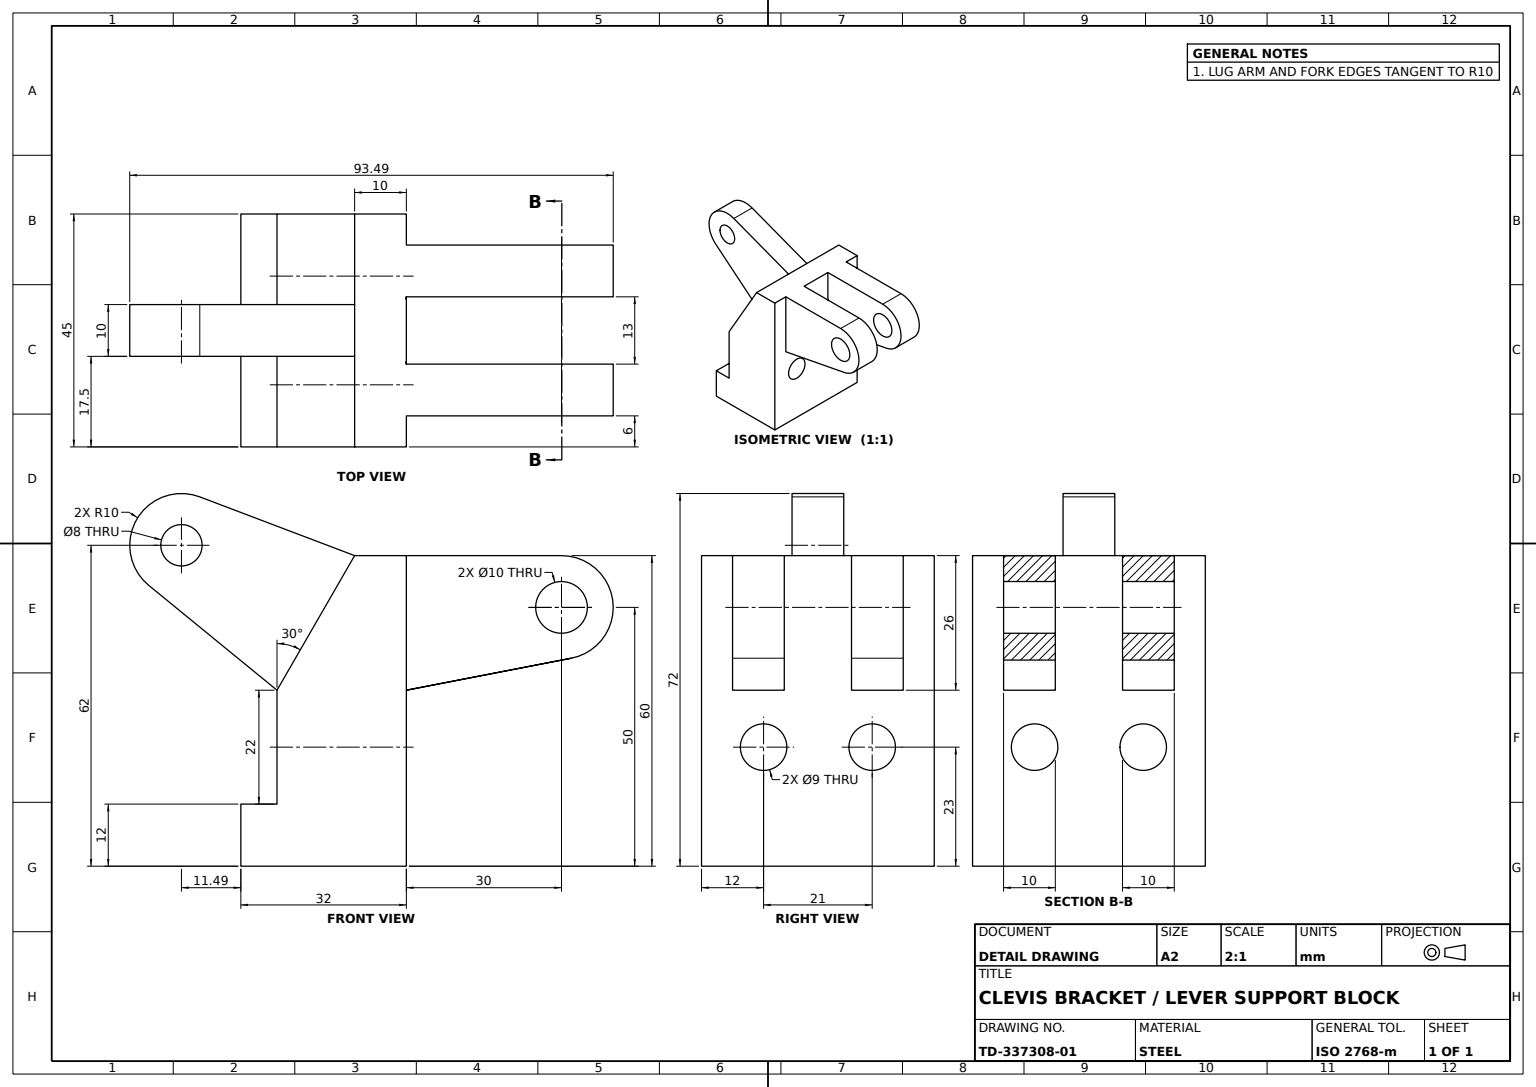
SolidWorks part; units mm, degrees
material "Plain Carbon Steel"
ref_plane "Front Plane" through (0, 0, 0) normal (0, 0, 1) x (1, 0, 0)
ref_plane "Top Plane" through (0, 0, 0) normal (0, 1, 0) x (1, 0, 0)
ref_plane "Right Plane" through (0, 0, 0) normal (1, 0, 0) x (0, 0, -1)
sketch "Base Block Profile Sketch" plane through (0, 0, 0) normal (0, 0, 1) x (1, 0, 0)
  line L0 (0, 0) -> (-32, 0)
  line L1 (-32, 0) -> (-32, 12)
  line L2 (-32, 12) -> (-25.0111, 12)
  line L3 (-25.0111, 12) -> (-25.0111, 34)
  line L4 (-25.0111, 34) -> (-10, 60)
  line L5 (-10, 60) -> (0, 60)
  line L6 (0, 60) -> (0, 0)
  dimension "D1" = 10
  dimension "D2" = 60
  dimension "D3" = 32
  dimension "D4" = 12
  dimension "D5" = 22
  dimension "D6" = 30
extrude "Base Block" add sketch "Base Block Profile Sketch" along normal mid plane 45
sketch "Lug Arm Sketch" plane through (0, 0, 0) normal (0, 0, 1) x (1, 0, 0)
  line L0 (-25.0111, 34) -> (-49.8118, 54.2548)
  line L1 (-43.4863, 62) -> (-17.5056, 47) construction
  line L2 (-10, 60) -> (-25.0111, 34) construction
  line L3 (-39.9415, 71.3506) -> (-10, 60)
  line L4 (-25.0111, 34) -> (-10, 60)
  arc A0 (-39.9415, 71.3506) -> (-49.8118, 54.2548) centre (-43.4863, 62) ccw
  circle A1 centre (-43.4863, 62) radius 4
  point P5 (-17.5056, 47)
  dimension "D2" = 8
  dimension "D3" = 10
  dimension "D1" = 30
extrude "Lug Arm" add sketch "Lug Arm Sketch" along normal mid plane 10
sketch "Side Hole Sketch" plane through (-25.0111, 0, 0) normal (-1, 0, 0) x (0, 0, 1)
  line L0 (22.5, 34) -> (22.5, 12) construction
  circle A0 centre (10.5, 23) radius 4.5
  circle A1 centre (-10.5, 23) radius 4.5
  point P8 (22.5, 23)
  dimension "D1" = 9
  dimension "D2" = 21
  dimension "D3" = 10.5
extrude "Side Hole Ø9" cut sketch "Side Hole Sketch" against normal up to next
sketch "Clevis Fork Sketch" plane through (0, 0, 22.5) normal (0, 0, 1) x (1, 0, 0)
  line L0 (0, 60) -> (30, 60)
  line L1 (0, 34) -> (31.9026, 40.1827)
  line L2 (0, 0) -> (0, 60) construction
  line L3 (0, 60) -> (0, 34)
  arc A0 (31.9026, 40.1827) -> (30, 60) centre (30, 50) ccw
  circle A1 centre (30, 50) radius 5
  dimension "D1" = 20
  dimension "D3" = 10
  dimension "D2" = 26
  dimension "D4" = 30
extrude "Clevis Fork" add sketch "Clevis Fork Sketch" against normal up to surface (45 mm away) up to face at (-17.7175, 25.4286, -22.5)
sketch "Clevis Pin Hole Sketch" plane through (0, 60, 0) normal (0, 1, 0) x (1, 0, 0)
  line L0 (0, 22.5) -> (0, -22.5) construction
  line L1 (0, -16.5) -> (40, -16.5)
  line L2 (0, -16.5) -> (0, -22.5)
  line L3 (0, -22.5) -> (40, -22.5)
  line L4 (40, -16.5) -> (40, -22.5)
  line L5 (40, -22.5) -> (40, 22.5) construction
  line L6 (30, -22.5) -> (-10, -22.5) construction
  line L7 (0, -6.5) -> (40, -6.5)
  line L8 (0, -6.5) -> (0, 6.5)
  line L9 (0, 6.5) -> (40, 6.5)
  line L10 (40, -6.5) -> (40, 6.5)
  line L11 (0, 16.5) -> (40, 16.5)
  line L12 (0, 16.5) -> (0, 22.5)
  line L13 (0, 22.5) -> (40, 22.5)
  line L14 (40, 16.5) -> (40, 22.5)
  point P17 (40, 0)
  dimension "D1" = 6
  dimension "D2" = 13
extrude "Clevis Pin Holes Ø6" cut sketch "Clevis Pin Hole Sketch" against normal through all
